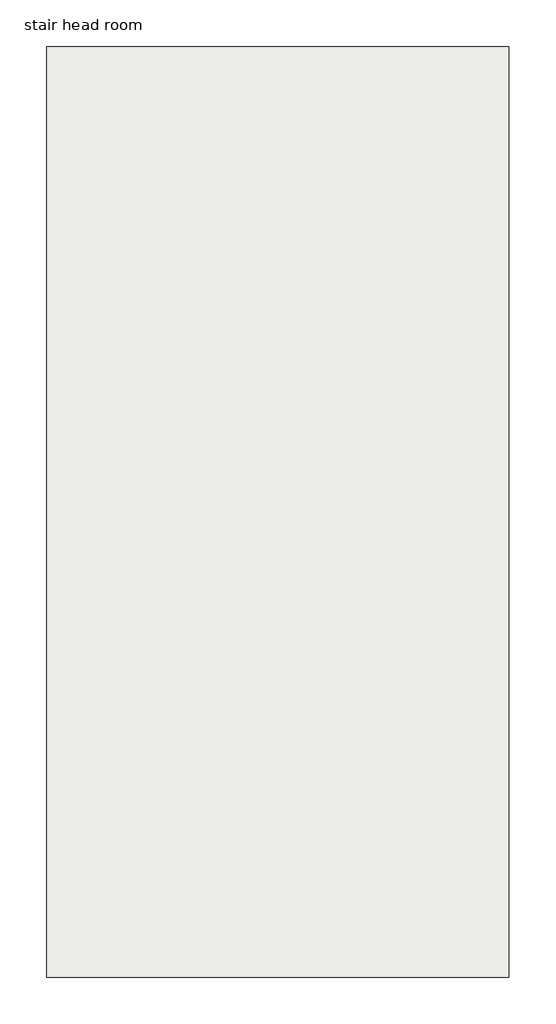
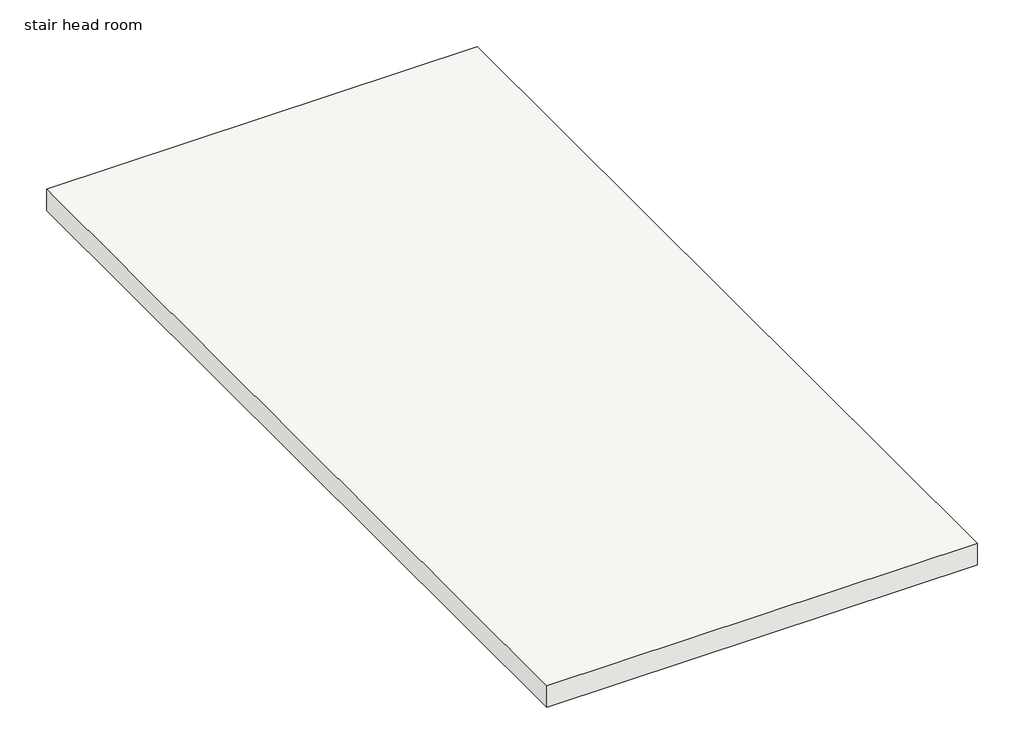
# One storey: 1 slab.
"""IFC4 building model written with IfcOpenShell, lengths in millimetres."""

from ifc_helpers import new_model, si_unit, frame, origin, place, context, project, spatial, polyline, outline, extrude, element, save

model = new_model("IFC4")

# Units and contexts
model_context = context("Model", 3, world=origin())
ifc_project = project(units=[si_unit("LENGTHUNIT", "METRE", prefix="MILLI")], contexts=[model_context])

# Site, building, storey
site = spatial("IfcSite", under=ifc_project)
building = spatial("IfcBuilding", under=site)
storey = spatial("IfcBuildingStorey", under=building, Name="stair head room", Elevation=7315.2)

# Slab
placement = place(None, origin())
element("IfcSlab", 1, ObjectType="Generic - 6\" -6", at=placement, inside=storey, context=model_context, shape_type="SweptSolid", body=[
    extrude(outline(polyline([(-5005.6994093, 6877.2237487), (-5005.6994093, 1047.9237487), (-7901.2994093, 1047.9237487), (-7901.2994093, 6877.2237487), (-5005.6994093, 6877.2237487)])), frame((0.0, 0.0, 7162.8), z_axis=(0.0, 0.0, 1.0), x_axis=(1.0, 0.0, 0.0)), (0.0, 0.0, 1.0), 152.4),
])

save(model, "model.ifc")

# Revit data of these elements
# Type "Generic - 6\" -6"
#   Assembly Code = "B1010"
#   Function = 0
#   Layers, outside or top first: 0' - 6" "Asphalt, Pavement, Light Grey" (function 1)
# Element 1 (IfcSlab, "Generic - 6\" -6")
#   Height Offset From Level = 0' - 0"
#   Phase Created = New Construction
#   Materials on its faces: "Asphalt, Pavement, Light Grey"
# Materials
#   "Asphalt, Pavement, Light Grey": class "Generic", colour RGB 120 120 120, transparency 0, Description = "Asphalt or tarmac paving", Cost = 0
